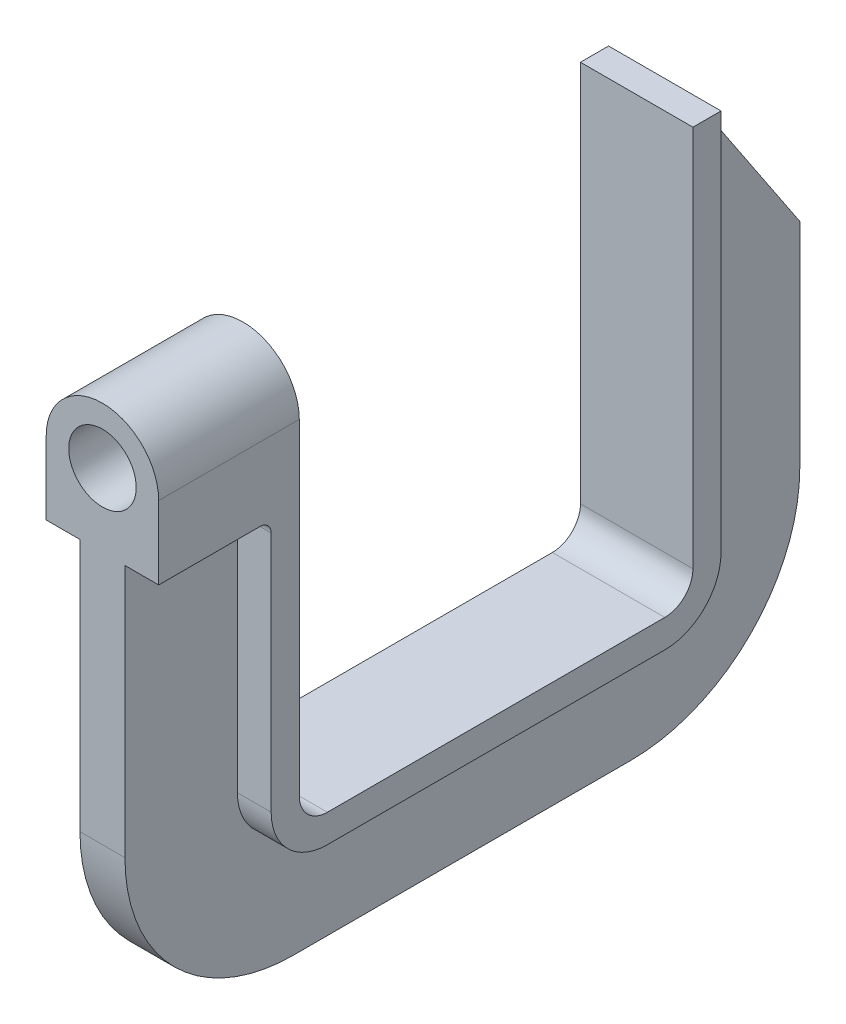
ISO-10303-21;
HEADER;
FILE_DESCRIPTION(('STEP AP214'),'2;1');
FILE_NAME('part.step','',(''),(''),'','','');
FILE_SCHEMA(('AUTOMOTIVE_DESIGN { 1 0 10303 214 1 1 1 1 }'));
ENDSEC;
DATA;
#1=APPLICATION_CONTEXT('core data for automotive mechanical design processes');
#2=APPLICATION_PROTOCOL_DEFINITION('international standard','automotive_design',2000,#1);
#3=PRODUCT_CONTEXT('',#1,'mechanical');
#4=PRODUCT('Part','Part','',(#3));
#5=PRODUCT_RELATED_PRODUCT_CATEGORY('part','',(#4));
#6=PRODUCT_DEFINITION_FORMATION('','',#4);
#7=PRODUCT_DEFINITION_CONTEXT('part definition',#1,'design');
#8=PRODUCT_DEFINITION('design','',#6,#7);
#9=PRODUCT_DEFINITION_SHAPE('','',#8);
#10=(LENGTH_UNIT() NAMED_UNIT(*) SI_UNIT(.MILLI.,.METRE.));
#11=(NAMED_UNIT(*) PLANE_ANGLE_UNIT() SI_UNIT($,.RADIAN.));
#12=(NAMED_UNIT(*) SI_UNIT($,.STERADIAN.) SOLID_ANGLE_UNIT());
#13=UNCERTAINTY_MEASURE_WITH_UNIT(LENGTH_MEASURE(1.E-05),#10,'distance_accuracy_value','');
#14=(GEOMETRIC_REPRESENTATION_CONTEXT(3) GLOBAL_UNCERTAINTY_ASSIGNED_CONTEXT((#13)) GLOBAL_UNIT_ASSIGNED_CONTEXT((#10,
#11,#12)) REPRESENTATION_CONTEXT('',''));
#15=CARTESIAN_POINT('',(0.,0.,0.));
#16=DIRECTION('',(0.,0.,1.));
#17=DIRECTION('',(1.,0.,0.));
#18=AXIS2_PLACEMENT_3D('',#15,#16,#17);
#19=CARTESIAN_POINT('',(4.,30.,-30.));
#20=DIRECTION('',(-1.,0.,0.));
#21=DIRECTION('',(0.,0.,1.));
#22=AXIS2_PLACEMENT_3D('',#19,#20,#21);
#23=PLANE('',#22);
#24=DIRECTION('',(0.,-1.,0.));
#25=VECTOR('',#24,1.);
#26=CARTESIAN_POINT('',(4.,30.,-20.));
#27=LINE('',#26,#25);
#28=CARTESIAN_POINT('',(4.,73.,-20.));
#29=VERTEX_POINT('',#28);
#30=CARTESIAN_POINT('',(4.,30.,-20.));
#31=VERTEX_POINT('',#30);
#32=EDGE_CURVE('E359',#29,#31,#27,.T.);
#33=ORIENTED_EDGE('',*,*,#32,.F.);
#34=CARTESIAN_POINT('',(4.,73.,-18.));
#35=DIRECTION('',(-1.,0.,0.));
#36=DIRECTION('',(0.,0.,1.));
#37=AXIS2_PLACEMENT_3D('',#34,#35,#36);
#38=CIRCLE('',#37,2.);
#39=CARTESIAN_POINT('',(4.,75.,-18.));
#40=VERTEX_POINT('',#39);
#41=EDGE_CURVE('E69',#29,#40,#38,.F.);
#42=ORIENTED_EDGE('',*,*,#41,.T.);
#43=DIRECTION('',(0.,0.,1.));
#44=VECTOR('',#43,1.);
#45=CARTESIAN_POINT('',(4.,75.,2.57268674916443E-13));
#46=LINE('',#45,#44);
#47=CARTESIAN_POINT('',(4.,75.,0.));
#48=VERTEX_POINT('',#47);
#49=EDGE_CURVE('E363',#40,#48,#46,.T.);
#50=ORIENTED_EDGE('',*,*,#49,.T.);
#51=DIRECTION('',(0.,-1.,0.));
#52=VECTOR('',#51,1.);
#53=CARTESIAN_POINT('',(4.,75.,2.57268674916443E-13));
#54=LINE('',#53,#52);
#55=CARTESIAN_POINT('',(4.,30.0000000000001,1.02907469966577E-13));
#56=VERTEX_POINT('',#55);
#57=EDGE_CURVE('E361',#48,#56,#54,.T.);
#58=ORIENTED_EDGE('',*,*,#57,.T.);
#59=CARTESIAN_POINT('',(4.,30.,-29.9999999999999));
#60=DIRECTION('',(1.,0.,0.));
#61=DIRECTION('',(0.,0.,-1.));
#62=AXIS2_PLACEMENT_3D('',#59,#60,#61);
#63=CIRCLE('',#62,30.);
#64=CARTESIAN_POINT('',(4.,0.,-30.0000000000001));
#65=VERTEX_POINT('',#64);
#66=EDGE_CURVE('E368',#56,#65,#63,.T.);
#67=ORIENTED_EDGE('',*,*,#66,.T.);
#68=DIRECTION('',(0.,0.,-1.));
#69=VECTOR('',#68,1.);
#70=CARTESIAN_POINT('',(4.,0.,-30.0000000000001));
#71=LINE('',#70,#69);
#72=CARTESIAN_POINT('',(4.,0.,-89.9999999999998));
#73=VERTEX_POINT('',#72);
#74=EDGE_CURVE('E366',#65,#73,#71,.T.);
#75=ORIENTED_EDGE('',*,*,#74,.T.);
#76=CARTESIAN_POINT('',(4.,30.,-90.));
#77=DIRECTION('',(1.,0.,0.));
#78=DIRECTION('',(0.,0.,-1.));
#79=AXIS2_PLACEMENT_3D('',#76,#77,#78);
#80=CIRCLE('',#79,30.);
#81=CARTESIAN_POINT('',(4.,30.,-120.));
#82=VERTEX_POINT('',#81);
#83=EDGE_CURVE('E367',#73,#82,#80,.T.);
#84=ORIENTED_EDGE('',*,*,#83,.T.);
#85=DIRECTION('',(0.,1.,0.));
#86=VECTOR('',#85,1.);
#87=CARTESIAN_POINT('',(4.,30.0000000000002,-120.));
#88=LINE('',#87,#86);
#89=CARTESIAN_POINT('',(4.,68.,-120.));
#90=VERTEX_POINT('',#89);
#91=EDGE_CURVE('E375',#82,#90,#88,.T.);
#92=ORIENTED_EDGE('',*,*,#91,.T.);
#93=DIRECTION('',(0.,0.832050294337843,0.554700196225229));
#94=VECTOR('',#93,1.);
#95=CARTESIAN_POINT('',(4.,68.,-120.));
#96=LINE('',#95,#94);
#97=CARTESIAN_POINT('',(4.,98.,-100.));
#98=VERTEX_POINT('',#97);
#99=EDGE_CURVE('E372',#90,#98,#96,.T.);
#100=ORIENTED_EDGE('',*,*,#99,.T.);
#101=DIRECTION('',(0.,1.,0.));
#102=VECTOR('',#101,1.);
#103=CARTESIAN_POINT('',(4.,30.,-100.));
#104=LINE('',#103,#102);
#105=CARTESIAN_POINT('',(4.,30.0000000000001,-100.));
#106=VERTEX_POINT('',#105);
#107=EDGE_CURVE('E347',#106,#98,#104,.T.);
#108=ORIENTED_EDGE('',*,*,#107,.F.);
#109=CARTESIAN_POINT('',(4.,30.,-90.));
#110=DIRECTION('',(-1.,0.,0.));
#111=DIRECTION('',(0.,0.,1.));
#112=AXIS2_PLACEMENT_3D('',#109,#110,#111);
#113=CIRCLE('',#112,10.);
#114=CARTESIAN_POINT('',(4.,20.,-89.9999999999999));
#115=VERTEX_POINT('',#114);
#116=EDGE_CURVE('E349',#115,#106,#113,.F.);
#117=ORIENTED_EDGE('',*,*,#116,.F.);
#118=DIRECTION('',(0.,0.,-1.));
#119=VECTOR('',#118,1.);
#120=CARTESIAN_POINT('',(4.,20.,-30.));
#121=LINE('',#120,#119);
#122=CARTESIAN_POINT('',(4.,20.,-30.));
#123=VERTEX_POINT('',#122);
#124=EDGE_CURVE('E355',#123,#115,#121,.T.);
#125=ORIENTED_EDGE('',*,*,#124,.F.);
#126=CARTESIAN_POINT('',(4.,30.,-30.));
#127=DIRECTION('',(-1.,0.,0.));
#128=DIRECTION('',(0.,0.,1.));
#129=AXIS2_PLACEMENT_3D('',#126,#127,#128);
#130=CIRCLE('',#129,10.);
#131=EDGE_CURVE('E354',#31,#123,#130,.F.);
#132=ORIENTED_EDGE('',*,*,#131,.F.);
#133=EDGE_LOOP('',(#33,#42,#50,#58,#67,#75,#84,#92,#100,#108,#117,#125,#132));
#134=FACE_BOUND('',#133,.T.);
#135=ADVANCED_FACE('F44',(#134),#23,.F.);
#136=CARTESIAN_POINT('',(-4.,30.,-30.));
#137=DIRECTION('',(-1.,0.,0.));
#138=DIRECTION('',(0.,0.,1.));
#139=AXIS2_PLACEMENT_3D('',#136,#137,#138);
#140=PLANE('',#139);
#141=DIRECTION('',(0.,0.,1.));
#142=VECTOR('',#141,1.);
#143=CARTESIAN_POINT('',(-4.,75.,2.57268674916443E-13));
#144=LINE('',#143,#142);
#145=CARTESIAN_POINT('',(-4.,75.,-18.));
#146=VERTEX_POINT('',#145);
#147=CARTESIAN_POINT('',(-4.,75.,0.));
#148=VERTEX_POINT('',#147);
#149=EDGE_CURVE('E358',#146,#148,#144,.T.);
#150=ORIENTED_EDGE('',*,*,#149,.F.);
#151=CARTESIAN_POINT('',(-4.,73.,-18.));
#152=DIRECTION('',(-1.,0.,0.));
#153=DIRECTION('',(0.,0.,1.));
#154=AXIS2_PLACEMENT_3D('',#151,#152,#153);
#155=CIRCLE('',#154,2.);
#156=CARTESIAN_POINT('',(-4.,73.,-20.));
#157=VERTEX_POINT('',#156);
#158=EDGE_CURVE('E437',#146,#157,#155,.T.);
#159=ORIENTED_EDGE('',*,*,#158,.T.);
#160=DIRECTION('',(0.,-1.,0.));
#161=VECTOR('',#160,1.);
#162=CARTESIAN_POINT('',(-4.,30.,-20.));
#163=LINE('',#162,#161);
#164=CARTESIAN_POINT('',(-4.,30.0000000000001,-20.));
#165=VERTEX_POINT('',#164);
#166=EDGE_CURVE('E427',#157,#165,#163,.T.);
#167=ORIENTED_EDGE('',*,*,#166,.T.);
#168=CARTESIAN_POINT('',(-4.,30.,-30.));
#169=DIRECTION('',(-1.,0.,0.));
#170=DIRECTION('',(0.,0.,1.));
#171=AXIS2_PLACEMENT_3D('',#168,#169,#170);
#172=CIRCLE('',#171,10.);
#173=CARTESIAN_POINT('',(-4.,20.,-30.));
#174=VERTEX_POINT('',#173);
#175=EDGE_CURVE('E426',#165,#174,#172,.F.);
#176=ORIENTED_EDGE('',*,*,#175,.T.);
#177=DIRECTION('',(0.,0.,-1.));
#178=VECTOR('',#177,1.);
#179=CARTESIAN_POINT('',(-4.,20.,-30.));
#180=LINE('',#179,#178);
#181=CARTESIAN_POINT('',(-4.,20.,-89.9999999999999));
#182=VERTEX_POINT('',#181);
#183=EDGE_CURVE('E421',#174,#182,#180,.T.);
#184=ORIENTED_EDGE('',*,*,#183,.T.);
#185=CARTESIAN_POINT('',(-4.,30.,-90.));
#186=DIRECTION('',(-1.,0.,0.));
#187=DIRECTION('',(0.,0.,1.));
#188=AXIS2_PLACEMENT_3D('',#185,#186,#187);
#189=CIRCLE('',#188,10.);
#190=CARTESIAN_POINT('',(-4.,30.0000000000001,-100.));
#191=VERTEX_POINT('',#190);
#192=EDGE_CURVE('E419',#182,#191,#189,.F.);
#193=ORIENTED_EDGE('',*,*,#192,.T.);
#194=DIRECTION('',(0.,1.,0.));
#195=VECTOR('',#194,1.);
#196=CARTESIAN_POINT('',(-4.,30.,-100.));
#197=LINE('',#196,#195);
#198=CARTESIAN_POINT('',(-4.,98.,-100.));
#199=VERTEX_POINT('',#198);
#200=EDGE_CURVE('E417',#191,#199,#197,.T.);
#201=ORIENTED_EDGE('',*,*,#200,.T.);
#202=DIRECTION('',(0.,0.832050294337843,0.554700196225229));
#203=VECTOR('',#202,1.);
#204=CARTESIAN_POINT('',(-4.,68.,-120.));
#205=LINE('',#204,#203);
#206=CARTESIAN_POINT('',(-4.,68.,-120.));
#207=VERTEX_POINT('',#206);
#208=EDGE_CURVE('E365',#207,#199,#205,.T.);
#209=ORIENTED_EDGE('',*,*,#208,.F.);
#210=DIRECTION('',(0.,1.,0.));
#211=VECTOR('',#210,1.);
#212=CARTESIAN_POINT('',(-4.,30.0000000000002,-120.));
#213=LINE('',#212,#211);
#214=CARTESIAN_POINT('',(-4.,30.,-120.));
#215=VERTEX_POINT('',#214);
#216=EDGE_CURVE('E387',#215,#207,#213,.T.);
#217=ORIENTED_EDGE('',*,*,#216,.F.);
#218=CARTESIAN_POINT('',(-4.,30.,-90.));
#219=DIRECTION('',(1.,0.,0.));
#220=DIRECTION('',(0.,0.,-1.));
#221=AXIS2_PLACEMENT_3D('',#218,#219,#220);
#222=CIRCLE('',#221,30.);
#223=CARTESIAN_POINT('',(-4.,0.,-89.9999999999998));
#224=VERTEX_POINT('',#223);
#225=EDGE_CURVE('E383',#224,#215,#222,.T.);
#226=ORIENTED_EDGE('',*,*,#225,.F.);
#227=DIRECTION('',(0.,0.,-1.));
#228=VECTOR('',#227,1.);
#229=CARTESIAN_POINT('',(-4.,0.,-30.0000000000001));
#230=LINE('',#229,#228);
#231=CARTESIAN_POINT('',(-4.,0.,-30.0000000000001));
#232=VERTEX_POINT('',#231);
#233=EDGE_CURVE('E385',#232,#224,#230,.T.);
#234=ORIENTED_EDGE('',*,*,#233,.F.);
#235=CARTESIAN_POINT('',(-4.,30.,-29.9999999999999));
#236=DIRECTION('',(1.,0.,0.));
#237=DIRECTION('',(0.,0.,-1.));
#238=AXIS2_PLACEMENT_3D('',#235,#236,#237);
#239=CIRCLE('',#238,30.);
#240=CARTESIAN_POINT('',(-4.,30.0000000000001,1.02907469966577E-13));
#241=VERTEX_POINT('',#240);
#242=EDGE_CURVE('E379',#241,#232,#239,.T.);
#243=ORIENTED_EDGE('',*,*,#242,.F.);
#244=DIRECTION('',(0.,-1.,0.));
#245=VECTOR('',#244,1.);
#246=CARTESIAN_POINT('',(-4.,75.,2.57268674916443E-13));
#247=LINE('',#246,#245);
#248=EDGE_CURVE('E378',#148,#241,#247,.T.);
#249=ORIENTED_EDGE('',*,*,#248,.F.);
#250=EDGE_LOOP('',(#150,#159,#167,#176,#184,#193,#201,#209,#217,#226,#234,#243,#249));
#251=FACE_BOUND('',#250,.T.);
#252=ADVANCED_FACE('F463',(#251),#140,.T.);
#253=CARTESIAN_POINT('',(4.,75.,2.57268674916443E-13));
#254=DIRECTION('',(0.,0.,-1.));
#255=DIRECTION('',(0.,1.,0.));
#256=AXIS2_PLACEMENT_3D('',#253,#254,#255);
#257=PLANE('',#256);
#258=CARTESIAN_POINT('',(0.,88.,0.));
#259=DIRECTION('',(0.,0.,1.));
#260=DIRECTION('',(1.,0.,0.));
#261=AXIS2_PLACEMENT_3D('',#258,#259,#260);
#262=CIRCLE('',#261,6.);
#263=CARTESIAN_POINT('',(6.,88.,0.));
#264=VERTEX_POINT('',#263);
#265=EDGE_CURVE('E262',#264,#264,#262,.T.);
#266=ORIENTED_EDGE('',*,*,#265,.F.);
#267=EDGE_LOOP('',(#266));
#268=FACE_BOUND('',#267,.T.);
#269=ORIENTED_EDGE('',*,*,#248,.T.);
#270=DIRECTION('',(-1.,0.,0.));
#271=VECTOR('',#270,1.);
#272=CARTESIAN_POINT('',(4.,30.0000000000001,1.02907469966577E-13));
#273=LINE('',#272,#271);
#274=EDGE_CURVE('E411',#56,#241,#273,.T.);
#275=ORIENTED_EDGE('',*,*,#274,.F.);
#276=ORIENTED_EDGE('',*,*,#57,.F.);
#277=DIRECTION('',(1.,0.,0.));
#278=VECTOR('',#277,1.);
#279=CARTESIAN_POINT('',(-10.,75.,0.));
#280=LINE('',#279,#278);
#281=CARTESIAN_POINT('',(10.,75.,0.));
#282=VERTEX_POINT('',#281);
#283=EDGE_CURVE('E268',#48,#282,#280,.T.);
#284=ORIENTED_EDGE('',*,*,#283,.T.);
#285=DIRECTION('',(0.,1.,0.));
#286=VECTOR('',#285,1.);
#287=CARTESIAN_POINT('',(10.,75.,0.));
#288=LINE('',#287,#286);
#289=CARTESIAN_POINT('',(10.,88.,0.));
#290=VERTEX_POINT('',#289);
#291=EDGE_CURVE('E257',#282,#290,#288,.T.);
#292=ORIENTED_EDGE('',*,*,#291,.T.);
#293=CARTESIAN_POINT('',(0.,88.,0.));
#294=DIRECTION('',(0.,0.,1.));
#295=DIRECTION('',(1.,0.,0.));
#296=AXIS2_PLACEMENT_3D('',#293,#294,#295);
#297=CIRCLE('',#296,10.);
#298=CARTESIAN_POINT('',(-10.,88.,0.));
#299=VERTEX_POINT('',#298);
#300=EDGE_CURVE('E246',#290,#299,#297,.T.);
#301=ORIENTED_EDGE('',*,*,#300,.T.);
#302=DIRECTION('',(0.,-1.,0.));
#303=VECTOR('',#302,1.);
#304=CARTESIAN_POINT('',(-10.,88.,0.));
#305=LINE('',#304,#303);
#306=CARTESIAN_POINT('',(-10.,75.,0.));
#307=VERTEX_POINT('',#306);
#308=EDGE_CURVE('E264',#299,#307,#305,.T.);
#309=ORIENTED_EDGE('',*,*,#308,.T.);
#310=EDGE_CURVE('E269',#307,#148,#280,.T.);
#311=ORIENTED_EDGE('',*,*,#310,.T.);
#312=EDGE_LOOP('',(#269,#275,#276,#284,#292,#301,#309,#311));
#313=FACE_BOUND('',#312,.T.);
#314=ADVANCED_FACE('F522',(#268,#313),#257,.F.);
#315=CARTESIAN_POINT('',(4.,30.,-29.9999999999999));
#316=DIRECTION('',(-1.,0.,0.));
#317=DIRECTION('',(0.,0.,1.));
#318=AXIS2_PLACEMENT_3D('',#315,#316,#317);
#319=CYLINDRICAL_SURFACE('',#318,30.);
#320=ORIENTED_EDGE('',*,*,#242,.T.);
#321=DIRECTION('',(-1.,0.,0.));
#322=VECTOR('',#321,1.);
#323=CARTESIAN_POINT('',(4.,0.,-30.0000000000001));
#324=LINE('',#323,#322);
#325=EDGE_CURVE('E412',#65,#232,#324,.T.);
#326=ORIENTED_EDGE('',*,*,#325,.F.);
#327=ORIENTED_EDGE('',*,*,#66,.F.);
#328=ORIENTED_EDGE('',*,*,#274,.T.);
#329=EDGE_LOOP('',(#320,#326,#327,#328));
#330=FACE_BOUND('',#329,.T.);
#331=ADVANCED_FACE('F526',(#330),#319,.T.);
#332=CARTESIAN_POINT('',(4.,0.,-30.0000000000001));
#333=DIRECTION('',(0.,1.,0.));
#334=DIRECTION('',(0.,0.,1.));
#335=AXIS2_PLACEMENT_3D('',#332,#333,#334);
#336=PLANE('',#335);
#337=ORIENTED_EDGE('',*,*,#233,.T.);
#338=DIRECTION('',(-1.,0.,0.));
#339=VECTOR('',#338,1.);
#340=CARTESIAN_POINT('',(4.,0.,-89.9999999999998));
#341=LINE('',#340,#339);
#342=EDGE_CURVE('E406',#73,#224,#341,.T.);
#343=ORIENTED_EDGE('',*,*,#342,.F.);
#344=ORIENTED_EDGE('',*,*,#74,.F.);
#345=ORIENTED_EDGE('',*,*,#325,.T.);
#346=EDGE_LOOP('',(#337,#343,#344,#345));
#347=FACE_BOUND('',#346,.T.);
#348=ADVANCED_FACE('F535',(#347),#336,.F.);
#349=CARTESIAN_POINT('',(4.,30.,-90.));
#350=DIRECTION('',(-1.,0.,0.));
#351=DIRECTION('',(0.,0.,1.));
#352=AXIS2_PLACEMENT_3D('',#349,#350,#351);
#353=CYLINDRICAL_SURFACE('',#352,30.);
#354=ORIENTED_EDGE('',*,*,#225,.T.);
#355=DIRECTION('',(-1.,0.,0.));
#356=VECTOR('',#355,1.);
#357=CARTESIAN_POINT('',(4.,30.,-120.));
#358=LINE('',#357,#356);
#359=EDGE_CURVE('E403',#82,#215,#358,.T.);
#360=ORIENTED_EDGE('',*,*,#359,.F.);
#361=ORIENTED_EDGE('',*,*,#83,.F.);
#362=ORIENTED_EDGE('',*,*,#342,.T.);
#363=EDGE_LOOP('',(#354,#360,#361,#362));
#364=FACE_BOUND('',#363,.T.);
#365=ADVANCED_FACE('F540',(#364),#353,.T.);
#366=CARTESIAN_POINT('',(4.,30.0000000000002,-120.));
#367=DIRECTION('',(0.,0.,1.));
#368=DIRECTION('',(1.,0.,0.));
#369=AXIS2_PLACEMENT_3D('',#366,#367,#368);
#370=PLANE('',#369);
#371=ORIENTED_EDGE('',*,*,#216,.T.);
#372=DIRECTION('',(-1.,0.,0.));
#373=VECTOR('',#372,1.);
#374=CARTESIAN_POINT('',(4.,68.,-120.));
#375=LINE('',#374,#373);
#376=EDGE_CURVE('E405',#90,#207,#375,.T.);
#377=ORIENTED_EDGE('',*,*,#376,.F.);
#378=ORIENTED_EDGE('',*,*,#91,.F.);
#379=ORIENTED_EDGE('',*,*,#359,.T.);
#380=EDGE_LOOP('',(#371,#377,#378,#379));
#381=FACE_BOUND('',#380,.T.);
#382=ADVANCED_FACE('F541',(#381),#370,.F.);
#383=CARTESIAN_POINT('',(4.,68.,-120.));
#384=DIRECTION('',(0.,-0.554700196225229,0.832050294337844));
#385=DIRECTION('',(0.,-0.832050294337844,-0.554700196225229));
#386=AXIS2_PLACEMENT_3D('',#383,#384,#385);
#387=PLANE('',#386);
#388=ORIENTED_EDGE('',*,*,#208,.T.);
#389=DIRECTION('',(-1.,0.,0.));
#390=VECTOR('',#389,1.);
#391=CARTESIAN_POINT('',(4.,98.,-100.));
#392=LINE('',#391,#390);
#393=EDGE_CURVE('E396',#98,#199,#392,.T.);
#394=ORIENTED_EDGE('',*,*,#393,.F.);
#395=ORIENTED_EDGE('',*,*,#99,.F.);
#396=ORIENTED_EDGE('',*,*,#376,.T.);
#397=EDGE_LOOP('',(#388,#394,#395,#396));
#398=FACE_BOUND('',#397,.T.);
#399=ADVANCED_FACE('F495',(#398),#387,.F.);
#400=CARTESIAN_POINT('',(4.,98.,-95.));
#401=DIRECTION('',(0.,-1.,0.));
#402=DIRECTION('',(0.,0.,-1.));
#403=AXIS2_PLACEMENT_3D('',#400,#401,#402);
#404=PLANE('',#403);
#405=ORIENTED_EDGE('',*,*,#393,.T.);
#406=DIRECTION('',(-1.,0.,0.));
#407=VECTOR('',#406,1.);
#408=CARTESIAN_POINT('',(10.,98.,-100.));
#409=LINE('',#408,#407);
#410=CARTESIAN_POINT('',(-10.,98.,-100.));
#411=VERTEX_POINT('',#410);
#412=EDGE_CURVE('E300',#199,#411,#409,.T.);
#413=ORIENTED_EDGE('',*,*,#412,.T.);
#414=DIRECTION('',(0.,0.,1.));
#415=VECTOR('',#414,1.);
#416=CARTESIAN_POINT('',(-10.,98.,-95.));
#417=LINE('',#416,#415);
#418=CARTESIAN_POINT('',(-10.,98.,-95.));
#419=VERTEX_POINT('',#418);
#420=EDGE_CURVE('E311',#411,#419,#417,.T.);
#421=ORIENTED_EDGE('',*,*,#420,.T.);
#422=DIRECTION('',(-1.,0.,0.));
#423=VECTOR('',#422,1.);
#424=CARTESIAN_POINT('',(4.,98.,-95.));
#425=LINE('',#424,#423);
#426=CARTESIAN_POINT('',(10.,98.,-95.));
#427=VERTEX_POINT('',#426);
#428=EDGE_CURVE('E400',#427,#419,#425,.T.);
#429=ORIENTED_EDGE('',*,*,#428,.F.);
#430=DIRECTION('',(0.,0.,1.));
#431=VECTOR('',#430,1.);
#432=CARTESIAN_POINT('',(10.,98.,-95.));
#433=LINE('',#432,#431);
#434=CARTESIAN_POINT('',(10.,98.,-100.));
#435=VERTEX_POINT('',#434);
#436=EDGE_CURVE('E284',#435,#427,#433,.T.);
#437=ORIENTED_EDGE('',*,*,#436,.F.);
#438=EDGE_CURVE('E330',#435,#98,#409,.T.);
#439=ORIENTED_EDGE('',*,*,#438,.T.);
#440=EDGE_LOOP('',(#405,#413,#421,#429,#437,#439));
#441=FACE_BOUND('',#440,.T.);
#442=ADVANCED_FACE('F484',(#441),#404,.F.);
#443=CARTESIAN_POINT('',(4.,30.,-95.));
#444=DIRECTION('',(0.,0.,-1.));
#445=DIRECTION('',(0.,1.,0.));
#446=AXIS2_PLACEMENT_3D('',#443,#444,#445);
#447=PLANE('',#446);
#448=ORIENTED_EDGE('',*,*,#428,.T.);
#449=DIRECTION('',(0.,-1.,0.));
#450=VECTOR('',#449,1.);
#451=CARTESIAN_POINT('',(-10.,30.,-95.));
#452=LINE('',#451,#450);
#453=CARTESIAN_POINT('',(-10.,30.,-95.));
#454=VERTEX_POINT('',#453);
#455=EDGE_CURVE('E316',#419,#454,#452,.T.);
#456=ORIENTED_EDGE('',*,*,#455,.T.);
#457=DIRECTION('',(-1.,0.,0.));
#458=VECTOR('',#457,1.);
#459=CARTESIAN_POINT('',(4.,30.,-95.));
#460=LINE('',#459,#458);
#461=CARTESIAN_POINT('',(10.,30.,-95.));
#462=VERTEX_POINT('',#461);
#463=EDGE_CURVE('E394',#462,#454,#460,.T.);
#464=ORIENTED_EDGE('',*,*,#463,.F.);
#465=DIRECTION('',(0.,-1.,0.));
#466=VECTOR('',#465,1.);
#467=CARTESIAN_POINT('',(10.,30.,-95.));
#468=LINE('',#467,#466);
#469=EDGE_CURVE('E289',#427,#462,#468,.T.);
#470=ORIENTED_EDGE('',*,*,#469,.F.);
#471=EDGE_LOOP('',(#448,#456,#464,#470));
#472=FACE_BOUND('',#471,.T.);
#473=ADVANCED_FACE('F553',(#472),#447,.F.);
#474=CARTESIAN_POINT('',(4.,30.,-90.));
#475=DIRECTION('',(-1.,0.,0.));
#476=DIRECTION('',(0.,0.,1.));
#477=AXIS2_PLACEMENT_3D('',#474,#475,#476);
#478=CYLINDRICAL_SURFACE('',#477,5.);
#479=ORIENTED_EDGE('',*,*,#463,.T.);
#480=CARTESIAN_POINT('',(-10.,30.,-90.));
#481=DIRECTION('',(-1.,0.,0.));
#482=DIRECTION('',(0.,0.,1.));
#483=AXIS2_PLACEMENT_3D('',#480,#481,#482);
#484=CIRCLE('',#483,5.);
#485=CARTESIAN_POINT('',(-10.,25.,-90.));
#486=VERTEX_POINT('',#485);
#487=EDGE_CURVE('E317',#454,#486,#484,.T.);
#488=ORIENTED_EDGE('',*,*,#487,.T.);
#489=DIRECTION('',(-1.,0.,0.));
#490=VECTOR('',#489,1.);
#491=CARTESIAN_POINT('',(4.,25.,-90.));
#492=LINE('',#491,#490);
#493=CARTESIAN_POINT('',(10.,25.,-90.));
#494=VERTEX_POINT('',#493);
#495=EDGE_CURVE('E391',#494,#486,#492,.T.);
#496=ORIENTED_EDGE('',*,*,#495,.F.);
#497=CARTESIAN_POINT('',(10.,30.,-90.));
#498=DIRECTION('',(-1.,0.,0.));
#499=DIRECTION('',(0.,0.,1.));
#500=AXIS2_PLACEMENT_3D('',#497,#498,#499);
#501=CIRCLE('',#500,5.);
#502=EDGE_CURVE('E292',#462,#494,#501,.T.);
#503=ORIENTED_EDGE('',*,*,#502,.F.);
#504=EDGE_LOOP('',(#479,#488,#496,#503));
#505=FACE_BOUND('',#504,.T.);
#506=ADVANCED_FACE('F554',(#505),#478,.F.);
#507=CARTESIAN_POINT('',(4.,25.,-30.));
#508=DIRECTION('',(0.,-1.,0.));
#509=DIRECTION('',(0.,0.,-1.));
#510=AXIS2_PLACEMENT_3D('',#507,#508,#509);
#511=PLANE('',#510);
#512=ORIENTED_EDGE('',*,*,#495,.T.);
#513=DIRECTION('',(0.,0.,1.));
#514=VECTOR('',#513,1.);
#515=CARTESIAN_POINT('',(-10.,25.,-30.));
#516=LINE('',#515,#514);
#517=CARTESIAN_POINT('',(-10.,25.,-30.));
#518=VERTEX_POINT('',#517);
#519=EDGE_CURVE('E325',#486,#518,#516,.T.);
#520=ORIENTED_EDGE('',*,*,#519,.T.);
#521=DIRECTION('',(-1.,0.,0.));
#522=VECTOR('',#521,1.);
#523=CARTESIAN_POINT('',(4.,25.,-30.));
#524=LINE('',#523,#522);
#525=CARTESIAN_POINT('',(10.,25.,-30.));
#526=VERTEX_POINT('',#525);
#527=EDGE_CURVE('E393',#526,#518,#524,.T.);
#528=ORIENTED_EDGE('',*,*,#527,.F.);
#529=DIRECTION('',(0.,0.,1.));
#530=VECTOR('',#529,1.);
#531=CARTESIAN_POINT('',(10.,25.,-30.));
#532=LINE('',#531,#530);
#533=EDGE_CURVE('E294',#494,#526,#532,.T.);
#534=ORIENTED_EDGE('',*,*,#533,.F.);
#535=EDGE_LOOP('',(#512,#520,#528,#534));
#536=FACE_BOUND('',#535,.T.);
#537=ADVANCED_FACE('F549',(#536),#511,.F.);
#538=CARTESIAN_POINT('',(4.,30.,-30.));
#539=DIRECTION('',(-1.,0.,0.));
#540=DIRECTION('',(0.,0.,1.));
#541=AXIS2_PLACEMENT_3D('',#538,#539,#540);
#542=CYLINDRICAL_SURFACE('',#541,5.);
#543=ORIENTED_EDGE('',*,*,#527,.T.);
#544=CARTESIAN_POINT('',(-10.,30.,-30.));
#545=DIRECTION('',(-1.,0.,0.));
#546=DIRECTION('',(0.,0.,-1.));
#547=AXIS2_PLACEMENT_3D('',#544,#545,#546);
#548=CIRCLE('',#547,5.);
#549=CARTESIAN_POINT('',(-10.,30.,-25.));
#550=VERTEX_POINT('',#549);
#551=EDGE_CURVE('E243',#518,#550,#548,.T.);
#552=ORIENTED_EDGE('',*,*,#551,.T.);
#553=DIRECTION('',(-1.,0.,0.));
#554=VECTOR('',#553,1.);
#555=CARTESIAN_POINT('',(4.,30.,-25.));
#556=LINE('',#555,#554);
#557=CARTESIAN_POINT('',(10.,30.,-25.));
#558=VERTEX_POINT('',#557);
#559=EDGE_CURVE('E376',#558,#550,#556,.T.);
#560=ORIENTED_EDGE('',*,*,#559,.F.);
#561=CARTESIAN_POINT('',(10.,30.,-30.));
#562=DIRECTION('',(-1.,0.,0.));
#563=DIRECTION('',(0.,0.,-1.));
#564=AXIS2_PLACEMENT_3D('',#561,#562,#563);
#565=CIRCLE('',#564,5.);
#566=EDGE_CURVE('E240',#526,#558,#565,.T.);
#567=ORIENTED_EDGE('',*,*,#566,.F.);
#568=EDGE_LOOP('',(#543,#552,#560,#567));
#569=FACE_BOUND('',#568,.T.);
#570=ADVANCED_FACE('F550',(#569),#542,.F.);
#571=CARTESIAN_POINT('',(4.,75.,-25.));
#572=DIRECTION('',(0.,0.,1.));
#573=DIRECTION('',(0.,-1.,0.));
#574=AXIS2_PLACEMENT_3D('',#571,#572,#573);
#575=PLANE('',#574);
#576=CARTESIAN_POINT('',(0.,88.,-25.));
#577=DIRECTION('',(0.,0.,1.));
#578=DIRECTION('',(0.,-1.,0.));
#579=AXIS2_PLACEMENT_3D('',#576,#577,#578);
#580=CIRCLE('',#579,6.);
#581=CARTESIAN_POINT('',(0.,82.,-25.));
#582=VERTEX_POINT('',#581);
#583=EDGE_CURVE('E267',#582,#582,#580,.T.);
#584=ORIENTED_EDGE('',*,*,#583,.T.);
#585=EDGE_LOOP('',(#584));
#586=FACE_BOUND('',#585,.T.);
#587=ORIENTED_EDGE('',*,*,#559,.T.);
#588=DIRECTION('',(0.,1.,0.));
#589=VECTOR('',#588,1.);
#590=CARTESIAN_POINT('',(-10.,75.,-25.));
#591=LINE('',#590,#589);
#592=CARTESIAN_POINT('',(-10.,88.,-25.));
#593=VERTEX_POINT('',#592);
#594=EDGE_CURVE('E254',#550,#593,#591,.T.);
#595=ORIENTED_EDGE('',*,*,#594,.T.);
#596=CARTESIAN_POINT('',(0.,88.,-25.));
#597=DIRECTION('',(0.,0.,1.));
#598=DIRECTION('',(1.,0.,0.));
#599=AXIS2_PLACEMENT_3D('',#596,#597,#598);
#600=CIRCLE('',#599,10.);
#601=CARTESIAN_POINT('',(10.,88.,-25.));
#602=VERTEX_POINT('',#601);
#603=EDGE_CURVE('E250',#602,#593,#600,.T.);
#604=ORIENTED_EDGE('',*,*,#603,.F.);
#605=DIRECTION('',(0.,1.,0.));
#606=VECTOR('',#605,1.);
#607=CARTESIAN_POINT('',(10.,75.,-25.));
#608=LINE('',#607,#606);
#609=EDGE_CURVE('E227',#558,#602,#608,.T.);
#610=ORIENTED_EDGE('',*,*,#609,.F.);
#611=EDGE_LOOP('',(#587,#595,#604,#610));
#612=FACE_BOUND('',#611,.T.);
#613=ADVANCED_FACE('F251',(#586,#612),#575,.F.);
#614=CARTESIAN_POINT('',(-10.,30.,-30.));
#615=DIRECTION('',(1.,0.,0.));
#616=DIRECTION('',(0.,0.,-1.));
#617=AXIS2_PLACEMENT_3D('',#614,#615,#616);
#618=PLANE('',#617);
#619=ORIENTED_EDGE('',*,*,#594,.F.);
#620=ORIENTED_EDGE('',*,*,#551,.F.);
#621=ORIENTED_EDGE('',*,*,#519,.F.);
#622=ORIENTED_EDGE('',*,*,#487,.F.);
#623=ORIENTED_EDGE('',*,*,#455,.F.);
#624=ORIENTED_EDGE('',*,*,#420,.F.);
#625=DIRECTION('',(0.,1.,0.));
#626=VECTOR('',#625,1.);
#627=CARTESIAN_POINT('',(-10.,98.,-100.));
#628=LINE('',#627,#626);
#629=CARTESIAN_POINT('',(-10.,30.0000000000001,-100.));
#630=VERTEX_POINT('',#629);
#631=EDGE_CURVE('E309',#630,#411,#628,.T.);
#632=ORIENTED_EDGE('',*,*,#631,.F.);
#633=CARTESIAN_POINT('',(-10.,30.,-90.));
#634=DIRECTION('',(1.,0.,0.));
#635=DIRECTION('',(0.,0.,1.));
#636=AXIS2_PLACEMENT_3D('',#633,#634,#635);
#637=CIRCLE('',#636,10.);
#638=CARTESIAN_POINT('',(-10.,20.,-89.9999999999999));
#639=VERTEX_POINT('',#638);
#640=EDGE_CURVE('E307',#639,#630,#637,.T.);
#641=ORIENTED_EDGE('',*,*,#640,.F.);
#642=DIRECTION('',(0.,0.,-1.));
#643=VECTOR('',#642,1.);
#644=CARTESIAN_POINT('',(-10.,20.,-89.9999999999999));
#645=LINE('',#644,#643);
#646=CARTESIAN_POINT('',(-10.,20.,-30.));
#647=VERTEX_POINT('',#646);
#648=EDGE_CURVE('E301',#647,#639,#645,.T.);
#649=ORIENTED_EDGE('',*,*,#648,.F.);
#650=CARTESIAN_POINT('',(-10.,30.,-30.));
#651=DIRECTION('',(1.,0.,0.));
#652=DIRECTION('',(0.,0.,1.));
#653=AXIS2_PLACEMENT_3D('',#650,#651,#652);
#654=CIRCLE('',#653,10.);
#655=CARTESIAN_POINT('',(-10.,30.0000000000001,-20.));
#656=VERTEX_POINT('',#655);
#657=EDGE_CURVE('E302',#656,#647,#654,.T.);
#658=ORIENTED_EDGE('',*,*,#657,.F.);
#659=DIRECTION('',(0.,-1.,0.));
#660=VECTOR('',#659,1.);
#661=CARTESIAN_POINT('',(-10.,75.,-20.));
#662=LINE('',#661,#660);
#663=CARTESIAN_POINT('',(-10.,73.,-20.));
#664=VERTEX_POINT('',#663);
#665=EDGE_CURVE('E297',#664,#656,#662,.T.);
#666=ORIENTED_EDGE('',*,*,#665,.F.);
#667=CARTESIAN_POINT('',(-10.,73.,-18.));
#668=DIRECTION('',(1.,0.,0.));
#669=DIRECTION('',(0.,0.,-1.));
#670=AXIS2_PLACEMENT_3D('',#667,#668,#669);
#671=CIRCLE('',#670,2.);
#672=CARTESIAN_POINT('',(-10.,75.,-18.));
#673=VERTEX_POINT('',#672);
#674=EDGE_CURVE('E52',#664,#673,#671,.T.);
#675=ORIENTED_EDGE('',*,*,#674,.T.);
#676=DIRECTION('',(0.,0.,1.));
#677=VECTOR('',#676,1.);
#678=CARTESIAN_POINT('',(-10.,75.,-25.));
#679=LINE('',#678,#677);
#680=EDGE_CURVE('E260',#673,#307,#679,.T.);
#681=ORIENTED_EDGE('',*,*,#680,.T.);
#682=ORIENTED_EDGE('',*,*,#308,.F.);
#683=DIRECTION('',(0.,0.,1.));
#684=VECTOR('',#683,1.);
#685=CARTESIAN_POINT('',(-10.,88.,-25.));
#686=LINE('',#685,#684);
#687=EDGE_CURVE('E248',#593,#299,#686,.T.);
#688=ORIENTED_EDGE('',*,*,#687,.F.);
#689=EDGE_LOOP('',(#619,#620,#621,#622,#623,#624,#632,#641,#649,#658,#666,#675,#681,#682,#688));
#690=FACE_BOUND('',#689,.T.);
#691=ADVANCED_FACE('F450',(#690),#618,.F.);
#692=CARTESIAN_POINT('',(10.,98.,-100.));
#693=DIRECTION('',(0.,0.,1.));
#694=DIRECTION('',(0.,-1.,0.));
#695=AXIS2_PLACEMENT_3D('',#692,#693,#694);
#696=PLANE('',#695);
#697=ORIENTED_EDGE('',*,*,#200,.F.);
#698=DIRECTION('',(-1.,0.,0.));
#699=VECTOR('',#698,1.);
#700=CARTESIAN_POINT('',(10.,30.0000000000001,-100.));
#701=LINE('',#700,#699);
#702=EDGE_CURVE('E329',#191,#630,#701,.T.);
#703=ORIENTED_EDGE('',*,*,#702,.T.);
#704=ORIENTED_EDGE('',*,*,#631,.T.);
#705=ORIENTED_EDGE('',*,*,#412,.F.);
#706=EDGE_LOOP('',(#697,#703,#704,#705));
#707=FACE_BOUND('',#706,.T.);
#708=ADVANCED_FACE('F485',(#707),#696,.F.);
#709=CARTESIAN_POINT('',(10.,30.,-90.));
#710=DIRECTION('',(-1.,0.,0.));
#711=DIRECTION('',(0.,0.,1.));
#712=AXIS2_PLACEMENT_3D('',#709,#710,#711);
#713=CYLINDRICAL_SURFACE('',#712,10.);
#714=ORIENTED_EDGE('',*,*,#192,.F.);
#715=DIRECTION('',(-1.,0.,0.));
#716=VECTOR('',#715,1.);
#717=CARTESIAN_POINT('',(10.,20.,-89.9999999999999));
#718=LINE('',#717,#716);
#719=EDGE_CURVE('E331',#182,#639,#718,.T.);
#720=ORIENTED_EDGE('',*,*,#719,.T.);
#721=ORIENTED_EDGE('',*,*,#640,.T.);
#722=ORIENTED_EDGE('',*,*,#702,.F.);
#723=EDGE_LOOP('',(#714,#720,#721,#722));
#724=FACE_BOUND('',#723,.T.);
#725=ADVANCED_FACE('F477',(#724),#713,.T.);
#726=CARTESIAN_POINT('',(10.,20.,-89.9999999999999));
#727=DIRECTION('',(0.,1.,0.));
#728=DIRECTION('',(0.,0.,1.));
#729=AXIS2_PLACEMENT_3D('',#726,#727,#728);
#730=PLANE('',#729);
#731=ORIENTED_EDGE('',*,*,#183,.F.);
#732=DIRECTION('',(-1.,0.,0.));
#733=VECTOR('',#732,1.);
#734=CARTESIAN_POINT('',(10.,20.,-30.));
#735=LINE('',#734,#733);
#736=EDGE_CURVE('E336',#174,#647,#735,.T.);
#737=ORIENTED_EDGE('',*,*,#736,.T.);
#738=ORIENTED_EDGE('',*,*,#648,.T.);
#739=ORIENTED_EDGE('',*,*,#719,.F.);
#740=EDGE_LOOP('',(#731,#737,#738,#739));
#741=FACE_BOUND('',#740,.T.);
#742=ADVANCED_FACE('F478',(#741),#730,.F.);
#743=CARTESIAN_POINT('',(10.,30.,-30.));
#744=DIRECTION('',(-1.,0.,0.));
#745=DIRECTION('',(0.,0.,1.));
#746=AXIS2_PLACEMENT_3D('',#743,#744,#745);
#747=CYLINDRICAL_SURFACE('',#746,10.);
#748=ORIENTED_EDGE('',*,*,#175,.F.);
#749=DIRECTION('',(-1.,0.,0.));
#750=VECTOR('',#749,1.);
#751=CARTESIAN_POINT('',(10.,30.0000000000001,-20.));
#752=LINE('',#751,#750);
#753=EDGE_CURVE('E345',#165,#656,#752,.T.);
#754=ORIENTED_EDGE('',*,*,#753,.T.);
#755=ORIENTED_EDGE('',*,*,#657,.T.);
#756=ORIENTED_EDGE('',*,*,#736,.F.);
#757=EDGE_LOOP('',(#748,#754,#755,#756));
#758=FACE_BOUND('',#757,.T.);
#759=ADVANCED_FACE('F466',(#758),#747,.T.);
#760=CARTESIAN_POINT('',(10.,75.,-20.));
#761=DIRECTION('',(0.,0.,-1.));
#762=DIRECTION('',(0.,1.,0.));
#763=AXIS2_PLACEMENT_3D('',#760,#761,#762);
#764=PLANE('',#763);
#765=ORIENTED_EDGE('',*,*,#166,.F.);
#766=DIRECTION('',(-1.,0.,0.));
#767=VECTOR('',#766,1.);
#768=CARTESIAN_POINT('',(10.,73.,-20.));
#769=LINE('',#768,#767);
#770=EDGE_CURVE('E431',#157,#664,#769,.T.);
#771=ORIENTED_EDGE('',*,*,#770,.T.);
#772=ORIENTED_EDGE('',*,*,#665,.T.);
#773=ORIENTED_EDGE('',*,*,#753,.F.);
#774=EDGE_LOOP('',(#765,#771,#772,#773));
#775=FACE_BOUND('',#774,.T.);
#776=ADVANCED_FACE('F467',(#775),#764,.F.);
#777=DIRECTION('',(0.,-1.,0.));
#778=VECTOR('',#777,1.);
#779=CARTESIAN_POINT('',(10.,75.,-20.));
#780=LINE('',#779,#778);
#781=CARTESIAN_POINT('',(10.,73.,-20.));
#782=VERTEX_POINT('',#781);
#783=CARTESIAN_POINT('',(10.,30.0000000000001,-20.));
#784=VERTEX_POINT('',#783);
#785=EDGE_CURVE('E238',#782,#784,#780,.T.);
#786=ORIENTED_EDGE('',*,*,#785,.F.);
#787=DIRECTION('',(-1.,0.,0.));
#788=VECTOR('',#787,1.);
#789=CARTESIAN_POINT('',(10.,73.,-20.));
#790=LINE('',#789,#788);
#791=EDGE_CURVE('E439',#782,#29,#790,.T.);
#792=ORIENTED_EDGE('',*,*,#791,.T.);
#793=ORIENTED_EDGE('',*,*,#32,.T.);
#794=EDGE_CURVE('E344',#784,#31,#752,.T.);
#795=ORIENTED_EDGE('',*,*,#794,.F.);
#796=EDGE_LOOP('',(#786,#792,#793,#795));
#797=FACE_BOUND('',#796,.T.);
#798=ADVANCED_FACE('F515',(#797),#764,.F.);
#799=ORIENTED_EDGE('',*,*,#794,.T.);
#800=ORIENTED_EDGE('',*,*,#131,.T.);
#801=CARTESIAN_POINT('',(10.,20.,-30.));
#802=VERTEX_POINT('',#801);
#803=EDGE_CURVE('E337',#802,#123,#735,.T.);
#804=ORIENTED_EDGE('',*,*,#803,.F.);
#805=CARTESIAN_POINT('',(10.,30.,-30.));
#806=DIRECTION('',(1.,0.,0.));
#807=DIRECTION('',(0.,0.,1.));
#808=AXIS2_PLACEMENT_3D('',#805,#806,#807);
#809=CIRCLE('',#808,10.);
#810=EDGE_CURVE('E280',#784,#802,#809,.T.);
#811=ORIENTED_EDGE('',*,*,#810,.F.);
#812=EDGE_LOOP('',(#799,#800,#804,#811));
#813=FACE_BOUND('',#812,.T.);
#814=ADVANCED_FACE('F510',(#813),#747,.T.);
#815=ORIENTED_EDGE('',*,*,#803,.T.);
#816=ORIENTED_EDGE('',*,*,#124,.T.);
#817=CARTESIAN_POINT('',(10.,20.,-89.9999999999999));
#818=VERTEX_POINT('',#817);
#819=EDGE_CURVE('E333',#818,#115,#718,.T.);
#820=ORIENTED_EDGE('',*,*,#819,.F.);
#821=DIRECTION('',(0.,0.,-1.));
#822=VECTOR('',#821,1.);
#823=CARTESIAN_POINT('',(10.,20.,-89.9999999999999));
#824=LINE('',#823,#822);
#825=EDGE_CURVE('E276',#802,#818,#824,.T.);
#826=ORIENTED_EDGE('',*,*,#825,.F.);
#827=EDGE_LOOP('',(#815,#816,#820,#826));
#828=FACE_BOUND('',#827,.T.);
#829=ADVANCED_FACE('F501',(#828),#730,.F.);
#830=ORIENTED_EDGE('',*,*,#819,.T.);
#831=ORIENTED_EDGE('',*,*,#116,.T.);
#832=CARTESIAN_POINT('',(10.,30.0000000000001,-100.));
#833=VERTEX_POINT('',#832);
#834=EDGE_CURVE('E332',#833,#106,#701,.T.);
#835=ORIENTED_EDGE('',*,*,#834,.F.);
#836=CARTESIAN_POINT('',(10.,30.,-90.));
#837=DIRECTION('',(1.,0.,0.));
#838=DIRECTION('',(0.,0.,1.));
#839=AXIS2_PLACEMENT_3D('',#836,#837,#838);
#840=CIRCLE('',#839,10.);
#841=EDGE_CURVE('E283',#818,#833,#840,.T.);
#842=ORIENTED_EDGE('',*,*,#841,.F.);
#843=EDGE_LOOP('',(#830,#831,#835,#842));
#844=FACE_BOUND('',#843,.T.);
#845=ADVANCED_FACE('F499',(#844),#713,.T.);
#846=ORIENTED_EDGE('',*,*,#834,.T.);
#847=ORIENTED_EDGE('',*,*,#107,.T.);
#848=ORIENTED_EDGE('',*,*,#438,.F.);
#849=DIRECTION('',(0.,1.,0.));
#850=VECTOR('',#849,1.);
#851=CARTESIAN_POINT('',(10.,98.,-100.));
#852=LINE('',#851,#850);
#853=EDGE_CURVE('E281',#833,#435,#852,.T.);
#854=ORIENTED_EDGE('',*,*,#853,.F.);
#855=EDGE_LOOP('',(#846,#847,#848,#854));
#856=FACE_BOUND('',#855,.T.);
#857=ADVANCED_FACE('F493',(#856),#696,.F.);
#858=CARTESIAN_POINT('',(10.,30.,-30.));
#859=DIRECTION('',(1.,0.,0.));
#860=DIRECTION('',(0.,0.,-1.));
#861=AXIS2_PLACEMENT_3D('',#858,#859,#860);
#862=PLANE('',#861);
#863=ORIENTED_EDGE('',*,*,#609,.T.);
#864=DIRECTION('',(0.,0.,1.));
#865=VECTOR('',#864,1.);
#866=CARTESIAN_POINT('',(10.,88.,-25.));
#867=LINE('',#866,#865);
#868=EDGE_CURVE('E234',#602,#290,#867,.T.);
#869=ORIENTED_EDGE('',*,*,#868,.T.);
#870=ORIENTED_EDGE('',*,*,#291,.F.);
#871=DIRECTION('',(0.,0.,1.));
#872=VECTOR('',#871,1.);
#873=CARTESIAN_POINT('',(10.,75.,-25.));
#874=LINE('',#873,#872);
#875=CARTESIAN_POINT('',(10.,75.,-18.));
#876=VERTEX_POINT('',#875);
#877=EDGE_CURVE('E253',#876,#282,#874,.T.);
#878=ORIENTED_EDGE('',*,*,#877,.F.);
#879=CARTESIAN_POINT('',(10.,73.,-18.));
#880=DIRECTION('',(1.,0.,0.));
#881=DIRECTION('',(0.,0.,-1.));
#882=AXIS2_PLACEMENT_3D('',#879,#880,#881);
#883=CIRCLE('',#882,2.);
#884=EDGE_CURVE('E11',#876,#782,#883,.F.);
#885=ORIENTED_EDGE('',*,*,#884,.T.);
#886=ORIENTED_EDGE('',*,*,#785,.T.);
#887=ORIENTED_EDGE('',*,*,#810,.T.);
#888=ORIENTED_EDGE('',*,*,#825,.T.);
#889=ORIENTED_EDGE('',*,*,#841,.T.);
#890=ORIENTED_EDGE('',*,*,#853,.T.);
#891=ORIENTED_EDGE('',*,*,#436,.T.);
#892=ORIENTED_EDGE('',*,*,#469,.T.);
#893=ORIENTED_EDGE('',*,*,#502,.T.);
#894=ORIENTED_EDGE('',*,*,#533,.T.);
#895=ORIENTED_EDGE('',*,*,#566,.T.);
#896=EDGE_LOOP('',(#863,#869,#870,#878,#885,#886,#887,#888,#889,#890,#891,#892,#893,#894,#895));
#897=FACE_BOUND('',#896,.T.);
#898=ADVANCED_FACE('F232',(#897),#862,.T.);
#899=CARTESIAN_POINT('',(-10.,75.,-25.));
#900=DIRECTION('',(0.,-1.,0.));
#901=DIRECTION('',(0.,0.,-1.));
#902=AXIS2_PLACEMENT_3D('',#899,#900,#901);
#903=PLANE('',#902);
#904=ORIENTED_EDGE('',*,*,#49,.F.);
#905=DIRECTION('',(-1.,0.,0.));
#906=VECTOR('',#905,1.);
#907=CARTESIAN_POINT('',(-10.,75.,-18.));
#908=LINE('',#907,#906);
#909=EDGE_CURVE('E58',#40,#876,#908,.F.);
#910=ORIENTED_EDGE('',*,*,#909,.T.);
#911=ORIENTED_EDGE('',*,*,#877,.T.);
#912=ORIENTED_EDGE('',*,*,#283,.F.);
#913=EDGE_LOOP('',(#904,#910,#911,#912));
#914=FACE_BOUND('',#913,.T.);
#915=ADVANCED_FACE('F516',(#914),#903,.T.);
#916=CARTESIAN_POINT('',(0.,88.,-25.));
#917=DIRECTION('',(0.,0.,1.));
#918=DIRECTION('',(1.,0.,0.));
#919=AXIS2_PLACEMENT_3D('',#916,#917,#918);
#920=CYLINDRICAL_SURFACE('',#919,10.);
#921=ORIENTED_EDGE('',*,*,#300,.F.);
#922=ORIENTED_EDGE('',*,*,#868,.F.);
#923=ORIENTED_EDGE('',*,*,#603,.T.);
#924=ORIENTED_EDGE('',*,*,#687,.T.);
#925=EDGE_LOOP('',(#921,#922,#923,#924));
#926=FACE_BOUND('',#925,.T.);
#927=ADVANCED_FACE('F247',(#926),#920,.T.);
#928=ORIENTED_EDGE('',*,*,#680,.F.);
#929=DIRECTION('',(-1.,0.,0.));
#930=VECTOR('',#929,1.);
#931=CARTESIAN_POINT('',(-10.,75.,-18.));
#932=LINE('',#931,#930);
#933=EDGE_CURVE('E436',#673,#146,#932,.F.);
#934=ORIENTED_EDGE('',*,*,#933,.T.);
#935=ORIENTED_EDGE('',*,*,#149,.T.);
#936=ORIENTED_EDGE('',*,*,#310,.F.);
#937=EDGE_LOOP('',(#928,#934,#935,#936));
#938=FACE_BOUND('',#937,.T.);
#939=ADVANCED_FACE('F453',(#938),#903,.T.);
#940=CARTESIAN_POINT('',(0.,88.,-43.));
#941=DIRECTION('',(0.,0.,1.));
#942=DIRECTION('',(1.,0.,0.));
#943=AXIS2_PLACEMENT_3D('',#940,#941,#942);
#944=CYLINDRICAL_SURFACE('',#943,6.);
#945=ORIENTED_EDGE('',*,*,#265,.T.);
#946=EDGE_LOOP('',(#945));
#947=FACE_BOUND('',#946,.T.);
#948=ORIENTED_EDGE('',*,*,#583,.F.);
#949=EDGE_LOOP('',(#948));
#950=FACE_BOUND('',#949,.T.);
#951=ADVANCED_FACE('F607',(#947,#950),#944,.F.);
#952=CARTESIAN_POINT('',(10.,73.,-18.));
#953=DIRECTION('',(-1.,0.,0.));
#954=DIRECTION('',(0.,0.,1.));
#955=AXIS2_PLACEMENT_3D('',#952,#953,#954);
#956=CYLINDRICAL_SURFACE('',#955,2.);
#957=ORIENTED_EDGE('',*,*,#158,.F.);
#958=ORIENTED_EDGE('',*,*,#933,.F.);
#959=ORIENTED_EDGE('',*,*,#674,.F.);
#960=ORIENTED_EDGE('',*,*,#770,.F.);
#961=EDGE_LOOP('',(#957,#958,#959,#960));
#962=FACE_BOUND('',#961,.T.);
#963=ADVANCED_FACE('F456',(#962),#956,.F.);
#964=CARTESIAN_POINT('',(10.,73.,-18.));
#965=DIRECTION('',(-1.,0.,0.));
#966=DIRECTION('',(0.,0.,1.));
#967=AXIS2_PLACEMENT_3D('',#964,#965,#966);
#968=CYLINDRICAL_SURFACE('',#967,2.);
#969=ORIENTED_EDGE('',*,*,#884,.F.);
#970=ORIENTED_EDGE('',*,*,#909,.F.);
#971=ORIENTED_EDGE('',*,*,#41,.F.);
#972=ORIENTED_EDGE('',*,*,#791,.F.);
#973=EDGE_LOOP('',(#969,#970,#971,#972));
#974=FACE_BOUND('',#973,.T.);
#975=ADVANCED_FACE('F50',(#974),#968,.F.);
#976=CLOSED_SHELL('',(#135,#252,#314,#331,#348,#365,#382,#399,#442,#473,#506,#537,#570,#613,
#691,#708,#725,#742,#759,#776,#798,#814,#829,#845,#857,#898,#915,#927,#939,#951,#963,#975));
#977=MANIFOLD_SOLID_BREP('B2',#976);
#978=ADVANCED_BREP_SHAPE_REPRESENTATION('',(#18,#977),#14);
#979=SHAPE_DEFINITION_REPRESENTATION(#9,#978);
ENDSEC;
END-ISO-10303-21;
